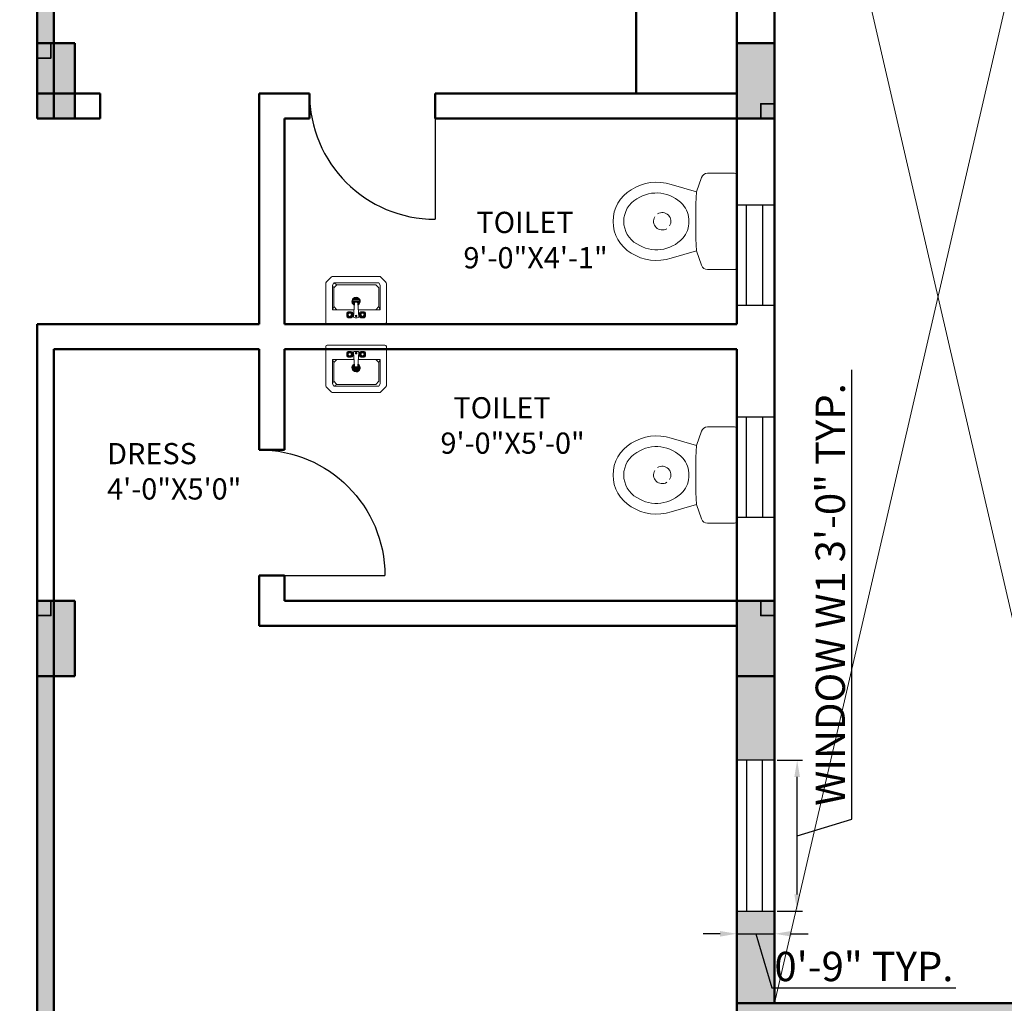
# Model space of a CAD drawing. Units: inches. Extents: x -7 to 1228, y -146 to 1091.
# Tile 63 of 88: x 376 to 611, y 655 to 890. Entities that reach past the tile are written whole.
import ezdxf

# ---------------------------------------------------------------- set-up
doc = ezdxf.new("R2010")
doc.units = ezdxf.units.IN
for name, color, linetype, lineweight in [('A-ANNO-DIMS', 2, 'Continuous', 18), ('A-AREA-IDEN', 7, 'Continuous', 18), ('A-COLS', 6, 'Continuous', 35), ('A-DOOR', 4, 'Continuous', 25), ('A-FLOR-FIXT', 8, 'Continuous', 18), ('A-FLOR-VOID', 7, 'Continuous', 18), ('A-FURN', 8, 'Continuous', 18), ('A-GLAZ', 175, 'Continuous', 25), ('A-WALL', 7, 'Continuous', 50), ('A-WALL-PATT', 251, 'Continuous', 13)]:
    doc.layers.add(name, color=color, linetype=linetype, lineweight=lineweight)
doc.styles.get("Standard").update_dxf_attribs({"font": 'arial.ttf'})
doc.dimstyles.new('ISO-25', dxfattribs={"dimtxt": 7, "dimasz": 4, "dimexe": 1.25, "dimexo": 0.625, "dimtad": 1, "dimdec": 1, "dimlunit": 3, "dimtxsty": 'Standard', "dimcen": 2.5, "dimadec": 0, "dimazin": 0, "dimtfac": 1, "dimtdec": 1, "dimtmove": 1, "dimatfit": 3, "dimfxl": 1, "dimarcsym": 0})

# ---------------------------------------------------------------- blocks, each defined once
blk = doc.blocks.new('A$C7B5C7CD4')
at = {"ltscale": 20}
for p, q in [((0, 0.614), (0, 0.4765)), ((0.243, 0.625), (0.011, 0.625)), ((0.243, 0.625), (0.475, 0.625)), ((0.486, 0.614), (0.486, 0.4765)), ((0.0212, 0.4467), (0.0946, 0.4214)), ((0.0946, 0.4214), (0.0576, 0.293)), ((0.0946, 0.4214), (0.1544, 0.4173)), ((0.3316, 0.4173), (0.1544, 0.4173)), ((0.3914, 0.4214), (0.3316, 0.4173)), ((0.4648, 0.4467), (0.3914, 0.4214)), ((0.3914, 0.4214), (0.4284, 0.293))]:
    blk.add_line(p, q, dxfattribs=at)
for centre, radius, start, end in [((0.011, 0.614), 0.011, 90, 180), ((0.475, 0.614), 0.011, 0, 90), ((0.0315, 0.4765), 0.0315, 180, 251), ((0.4545, 0.4765), 0.0315, 289, 0), ((0.2796, 0.219), 0.18, 132.4207, 213.289), ((0.24, 0.2602), 0.123, 88.6158, 131.7414), ((0.246, 0.2602), 0.123, 48.2586, 91.3842), ((0.2064, 0.219), 0.18, 326.711, 47.5793), ((0.2796, 0.219), 0.234, 161.5846, 212.8753), ((0.2064, 0.219), 0.234, 327.1247, 18.4154), ((0.243, 0.185), 0.131, 209.6292, 270), ((0.243, 0.185), 0.131, 270, 330.3708), ((0.243, 0.185), 0.185, 210.1745, 270), ((0.243, 0.185), 0.185, 270, 329.8255)]:
    blk.add_arc(centre, radius, start, end, dxfattribs=at)
for start, end in [(58.1785, 211.8215), (238.1785, 31.8215)]:
    blk.add_arc((0.2426, 0.2481), 0.0439, start, end)
blk = doc.blocks.new('A$C4CB854FF')
for p, q in [((0, 0.3675), (0, 0.0552)), ((0.4725, 0.38), (0.0125, 0.38)), ((0.1677, 0.2932), (0.1677, 0.318)), ((0.1745, 0.2919), (0.1745, 0.3194)), ((0.1773, 0.3221), (0.2048, 0.3221)), ((0.1787, 0.329), (0.2034, 0.329)), ((0.2075, 0.3194), (0.2075, 0.2919)), ((0.2144, 0.318), (0.2144, 0.2932)), ((0.2279, 0.2104), (0.2213, 0.3235)), ((0.2337, 0.329), (0.2502, 0.329)), ((0.2625, 0.3235), (0.256, 0.2104)), ((0.2694, 0.318), (0.2694, 0.2932)), ((0.2763, 0.3194), (0.2763, 0.2919)), ((0.3065, 0.3221), (0.279, 0.3221)), ((0.3052, 0.329), (0.2804, 0.329)), ((0.3093, 0.2919), (0.3093, 0.3194)), ((0.3162, 0.2932), (0.3162, 0.318)), ((0.485, 0.0552), (0.485, 0.3675)), ((0.05, 0.265), (0.2247, 0.265)), ((0.06, 0.24), (0.05, 0.265)), ((0.05, 0.07), (0.05, 0.265)), ((0.085, 0.265), (0.06, 0.24)), ((0.06, 0.24), (0.06, 0.09)), ((0.2048, 0.2891), (0.1773, 0.2891)), ((0.2034, 0.2822), (0.1787, 0.2822)), ((0.2591, 0.265), (0.43, 0.265)), ((0.279, 0.2891), (0.3065, 0.2891)), ((0.2804, 0.2822), (0.3052, 0.2822)), ((0.395, 0.265), (0.42, 0.24)), ((0.42, 0.24), (0.43, 0.265)), ((0.42, 0.24), (0.42, 0.09)), ((0.43, 0.07), (0.43, 0.265)), ((0.2152, 0.1984), (0.2694, 0.1984)), ((0.2297, 0.2066), (0.2165, 0.2066)), ((0.2681, 0.1901), (0.2165, 0.1901)), ((0.2272, 0.2149), (0.2208, 0.2149)), ((0.2638, 0.1819), (0.2208, 0.1819)), ((0.2533, 0.1736), (0.2313, 0.1736)), ((0.2505, 0.2052), (0.2334, 0.2052)), ((0.2681, 0.2066), (0.2541, 0.2066)), ((0.2638, 0.2149), (0.2566, 0.2149)), ((0.06, 0.09), (0.085, 0.065)), ((0.42, 0.09), (0.395, 0.065)), ((0.42, 0.09), (0.43, 0.07)), ((0.0037, 0.0463), (0.0463, 0.0037)), ((0.05, 0.07), (0.06, 0.05)), ((0.42, 0.05), (0.06, 0.05)), ((0.085, 0.065), (0.395, 0.065)), ((0.395, 0.065), (0.42, 0.05)), ((0.43, 0.07), (0.42, 0.05)), ((0.4387, 0.0037), (0.4813, 0.0463)), ((0.0552, 0), (0.4298, 0))]:
    blk.add_line(p, q)
for centre, radius in [((0.191, 0.3056), 0.0165), ((0.191, 0.3056), 0.0127), ((0.2419, 0.3152), 0.00688), ((0.2419, 0.3152), 0.00344), ((0.2928, 0.3056), 0.0165), ((0.2928, 0.3056), 0.0127)]:
    blk.add_circle(centre, radius)
for centre, radius, start, end in [((0.0125, 0.3675), 0.0125, 90, 180), ((0.1787, 0.318), 0.011, 90, 180), ((0.1773, 0.3194), 0.00275, 90, 180), ((0.2034, 0.318), 0.011, 0, 90), ((0.2048, 0.3194), 0.00275, 360, 90), ((0.2329, 0.314), 0.015, 87.19754, 140.72744), ((0.2509, 0.314), 0.015, 39.27256, 92.80246), ((0.2804, 0.318), 0.011, 90, 180), ((0.279, 0.3194), 0.00275, 90, 180), ((0.3052, 0.318), 0.011, 0, 90), ((0.3065, 0.3194), 0.00275, 360, 90), ((0.4725, 0.3675), 0.0125, 0, 90), ((0.1787, 0.2932), 0.011, 180, 270), ((0.1773, 0.2919), 0.00275, 180, 270), ((0.2034, 0.2932), 0.011, 270, 0), ((0.2048, 0.2919), 0.00275, 270, 0), ((0.2804, 0.2932), 0.011, 180, 270), ((0.279, 0.2919), 0.00275, 180, 270), ((0.3052, 0.2932), 0.011, 270, 360), ((0.3065, 0.2919), 0.00275, 270, 0), ((0.2423, 0.1984), 0.033, 118.68833, 62.86857), ((0.2423, 0.1984), 0.0271, 124.77581, 57.22467), ((0.2334, 0.2107), 0.0055, 183.3274, 270), ((0.2505, 0.2107), 0.0055, 270, 356.6726), ((0.0125, 0.0552), 0.0125, 180, 225), ((0.0552, 0.0125), 0.0125, 225, 270), ((0.4298, 0.0125), 0.0125, 270, 315), ((0.4725, 0.0552), 0.0125, 315, 0)]:
    blk.add_arc(centre, radius, start, end)
blk = doc.blocks.new('WIN-36')
for p, q in [((0, 36), (0, 0)), ((9, 36), (0, 36)), ((2.34, 36), (2.34, 0)), ((6.14, 0), (6.14, 36)), ((9, 0), (9, 36)), ((0, 0), (9, 0)), ((2.34, 0), (6.14, 0))]:
    blk.add_line(p, q)
blk = doc.blocks.new('WIN-24')
for p, q in [((0, 0), (0, 24)), ((0, 24), (9, 24)), ((2.34, 0), (2.34, 24)), ((2.34, 24), (6.14, 24)), ((6.14, 24), (6.14, 0)), ((9, 24), (9, 0)), ((9, 0), (0, 0))]:
    blk.add_line(p, q)
blk = doc.blocks.new('DOOR-750')
blk.add_line((30, 30), (30, 0))
blk.add_arc((30, 30), 30, 180, 270)
blk = doc.blocks.new('*D48')
at = {"layer": 'A-ANNO-DIMS', "color": 0, "lineweight": -2, "transparency": 16777216}
for p, q in [((574.46, 698.89), (574.46, 806.1)), ((556.62, 712.97), (562.65, 712.97)), ((561.4, 680.97), (561.4, 708.97)), ((561.4, 694.97), (574.46, 698.89)), ((556.62, 676.97), (562.65, 676.97))]:
    blk.add_line(p, q, dxfattribs=at)
at = {"layer": 'A-ANNO-DIMS', "color": 0, "transparency": 16777216}
for points in [[(560.73, 708.97), (562.07, 708.97), (561.4, 712.97)], [(560.73, 680.97), (562.07, 680.97), (561.4, 676.97)]]:
    blk.add_solid(points, dxfattribs=at)
at = {"layer": 'Defpoints', "color": 0, "transparency": 16777216}
for p in [(556, 712.97), (561.4, 712.97), (556, 676.97)]:
    blk.add_point(p, dxfattribs=at)
at = {"layer": 'A-ANNO-DIMS', "color": 0, "transparency": 16777216, "insert": (570.21, 752.49), "char_height": 7, "attachment_point": 5, "rotation": 90}
blk.add_mtext('WINDOW W1 3\'-0" TYP.', dxfattribs=at)
blk = doc.blocks.new('*D49')
at = {"layer": 'A-ANNO-DIMS', "color": 0, "lineweight": -2, "transparency": 16777216}
for p, q in [((547, 676.34), (547, 670.32)), ((556, 676.34), (556, 670.32)), ((543, 671.57), (539, 671.57)), ((547, 671.57), (556, 671.57)), ((547, 671.57), (556, 671.57)), ((551.5, 671.57), (555.37, 658.66)), ((560, 671.57), (564, 671.57)), ((555.37, 658.66), (599.29, 658.66))]:
    blk.add_line(p, q, dxfattribs=at)
at = {"layer": 'A-ANNO-DIMS', "color": 0, "transparency": 16777216}
for points in [[(543, 672.23), (543, 670.9), (547, 671.57)], [(560, 672.23), (560, 670.9), (556, 671.57)]]:
    blk.add_solid(points, dxfattribs=at)
at = {"layer": 'Defpoints', "color": 0, "transparency": 16777216}
for p in [(547, 676.97), (556, 676.97), (556, 671.57)]:
    blk.add_point(p, dxfattribs=at)
at = {"layer": 'A-ANNO-DIMS', "color": 0, "transparency": 16777216, "insert": (577.33, 662.86), "char_height": 7, "attachment_point": 5}
blk.add_mtext('0\'-9" TYP.', dxfattribs=at)

msp = doc.modelspace()

# ---------------------------------------------------------------- hatches: boundary and pattern name
at = {"layer": 'A-COLS'}
h = msp.add_hatch(color=256, dxfattribs=at)
h.dxf.hatch_style = 1
h.paths.add_polyline_path([(380, 866), (389, 866), (389, 884), (383.29, 884), (383.29, 880.45), (380, 880.45)])
h = msp.add_hatch(color=256, dxfattribs=at)
h.dxf.hatch_style = 1
h.paths.add_polyline_path([(383.29, 880.45), (383.29, 884), (380, 884), (380, 880.45)])
h = msp.add_hatch(color=256, dxfattribs=at)
h.dxf.hatch_style = 1
h.paths.add_polyline_path([(556, 884), (547, 884), (547, 866), (552.71, 866), (552.71, 869.55), (556, 869.55)])
h = msp.add_hatch(color=256, dxfattribs=at)
h.dxf.hatch_style = 1
h.paths.add_polyline_path([(552.71, 869.55), (552.71, 866), (556, 866), (556, 869.55)])
h = msp.add_hatch(color=256, dxfattribs=at)
h.dxf.hatch_style = 1
h.paths.add_polyline_path([(380, 733), (389, 733), (389, 751), (383.29, 751), (383.29, 747.45), (380, 747.45)])
h = msp.add_hatch(color=256, dxfattribs=at)
h.dxf.hatch_style = 1
h.paths.add_polyline_path([(383.29, 747.45), (383.29, 751), (380, 751), (380, 747.45)])
h = msp.add_hatch(color=256, dxfattribs=at)
h.dxf.hatch_style = 1
h.paths.add_polyline_path([(556, 747.45), (552.71, 747.45), (552.71, 751), (547, 751), (547, 733), (556, 733)])
h = msp.add_hatch(color=256, dxfattribs=at)
h.dxf.hatch_style = 1
h.paths.add_polyline_path([(556, 747.45), (556, 751), (552.71, 751), (552.71, 747.45)])
at = {"layer": 'A-WALL-PATT'}
h = msp.add_hatch(color=256, dxfattribs=at)
h.dxf.hatch_style = 1
h.paths.add_polyline_path([(69, 568), (60, 568), (60, 493), (63.29, 493), (69, 493)])
h.paths.add_polyline_path([(69, 662.41), (60, 662.41), (60, 586), (69, 586)], flags=17)
h.paths.add_polyline_path([(69, 723), (184, 723), (184, 734), (179, 734), (179, 728), (69, 728), (69, 741.62), (60, 741.62), (60, 698.41), (69, 698.41)], flags=17)
h.paths.add_polyline_path([(69, 782), (231, 782), (231, 728), (231, 723), (231, 586), (236, 586), (236, 787), (69, 787), (69, 800.13), (60, 800.13), (60, 765.62), (69, 765.62)])
h.paths.add_polyline_path([(184, 842), (189, 842), (189, 848), (173, 848), (173, 842), (179, 842), (179, 787), (184, 787)])
h.paths.add_polyline_path([(118.22, 69), (69, 69), (69, 60), (118.22, 60)])
h.paths.add_polyline_path([(227, 69), (154.22, 69), (154.22, 60), (227, 60)])
h.paths.add_polyline_path([(236, 60), (232.71, 60), (227, 60), (227, 36), (236, 36)])
h.paths.add_polyline_path([(389, 60), (380, 60), (380, 36), (389, 36)])
h.paths.add_polyline_path([(384, 181), (380, 181), (380, 115), (380, 78), (384, 78)])
h.paths.add_polyline_path([(380, 115), (334.55, 115), (334.55, 109), (380, 109)])
h.paths.add_polyline_path([(274.55, 115), (236, 115), (236, 201), (232.71, 201), (231, 201), (231, 78), (236, 78), (236, 109), (274.55, 109)])
h.paths.add_polyline_path([(69, 123), (60, 123), (60, 78), (69, 78)])
h.paths.add_polyline_path([(69, 201), (60, 201), (60, 159), (69, 159)])
h.paths.add_polyline_path([(143, 219), (69, 219), (69, 213), (143, 213)], flags=17)
h.paths.add_polyline_path([(189, 219), (184, 219), (184, 274), (231, 274), (231, 219), (236, 219), (236, 279), (184, 279), (184, 297), (179, 297), (179, 279), (69, 279), (69, 290.91), (60, 290.91), (60, 262.18), (69, 262.18), (69, 274), (179, 274), (179, 219), (173, 219), (173, 213), (189, 213)])
h.paths.add_polyline_path([(69, 238.18), (60, 238.18), (60, 219), (69, 219)], flags=17)
h.paths.add_polyline_path([(69, 333), (60, 333), (60, 314.91), (69, 314.91), (69, 316.96)])
h.paths.add_polyline_path([(190, 338), (184, 338), (69, 338), (69, 333), (179, 333), (179, 327), (184, 327), (184, 333.02), (190, 333.05)])
h.paths.add_polyline_path([(69, 386.81), (60, 386.81), (60, 351), (69, 351)])
h.paths.add_polyline_path([(69, 475), (60, 475), (60, 422.81), (69, 422.81)])
h.paths.add_polyline_path([(236, 475), (231, 475), (231, 351.24), (236, 351.24)])
h.paths.add_polyline_path([(384, 475), (380, 475), (380, 362), (384, 362)])
h.paths.add_polyline_path([(547, 307), (439, 307), (439, 356), (445, 356), (445, 362), (433, 362), (433, 307), (380, 307), (380, 244), (380, 241), (384, 241), (384, 301), (433, 301), (433, 277), (439, 277), (439, 301), (547, 301)])
h.paths.add_polyline_path([(547, 241), (439, 241), (439, 247), (433, 247), (433, 235), (547, 235)])
h.paths.add_polyline_path([(450, 69), (440.29, 69), (424.89, 69), (389, 69), (389, 60), (450, 60)])
h.paths.add_polyline_path([(547, 69), (486, 69), (486, 60), (547, 60)])
h.paths.add_polyline_path([(556, 148.27), (547, 148.27), (547, 78), (556, 78)])
h.paths.add_polyline_path([(556, 223), (547, 223), (547, 195), (547, 184.27), (556, 184.27)])
h.paths.add_polyline_path([(556, 311.19), (547, 311.19), (547, 273.08), (556, 273.08)])
h.paths.add_polyline_path([(556, 344), (552.71, 344), (547, 344), (547, 335.19), (556, 335.19)])
h.paths.add_polyline_path([(556, 249.08), (547, 249.08), (547, 241), (556, 241)])
h.paths.add_polyline_path([(547, 362), (475, 362), (475, 356), (547, 356)], flags=0)
h.paths.add_polyline_path([(556, 399.62), (547, 399.62), (547, 362), (556, 362)])
h.paths.add_polyline_path([(556, 475), (547, 475), (547, 435.62), (556, 435.62)])
h.paths.add_polyline_path([(547, 493), (389, 493), (389, 487), (547, 487)])
h.paths.add_polyline_path([(380, 493), (278, 493), (278, 487), (380, 487)])
h.paths.add_polyline_path([(227, 493), (69, 493), (69, 487), (227, 487)])
h.paths.add_polyline_path([(643, 122.44), (634, 122.44), (634, 78), (643, 78)])
h.paths.add_polyline_path([(702.5, 69), (692.79, 69), (677.39, 69), (643, 69), (643, 60), (702.5, 60)])
h.paths.add_polyline_path([(798, 69), (738.5, 69), (738.5, 60), (798, 60)])
h.paths.add_polyline_path([(807, 60), (803.71, 60), (798, 60), (798, 36), (807, 36)])
h.paths.add_polyline_path([(807, 109), (846.75, 109), (846.75, 115), (807, 115), (807, 159), (802, 159), (802, 78), (807, 78)])
h.paths.add_polyline_path([(807, 201), (802, 201), (802, 195), (807, 195)])
h.paths.add_polyline_path([(643, 201), (634, 201), (634, 158.44), (643, 158.44)])
h.paths.add_polyline_path([(756, 225), (751, 225), (751, 219), (643, 219), (643, 213), (756, 213)])
h.paths.add_polyline_path([(643, 240.85), (634, 240.85), (634, 219), (643, 219)])
h.paths.add_polyline_path([(643, 274), (643, 288.63), (634, 288.63), (634, 264.85), (643, 264.85)])
h.paths.add_polyline_path([(802, 279), (756, 279), (756, 297), (751, 297), (751, 279), (643, 279), (643, 274), (751, 274), (751, 255), (756, 255), (756, 274), (802, 274)])
h.paths.add_polyline_path([(807, 333), (803.71, 333), (802, 333), (802, 279), (802, 274), (802, 219), (807, 219)])
h.paths.add_polyline_path([(956, 182), (951, 182), (951, 115), (906.75, 115), (906.75, 109), (951, 109), (951, 78), (956, 78)])
h.paths.add_polyline_path([(960, 60), (951, 60), (951, 36), (960, 36)])
h.paths.add_polyline_path([(1021, 69), (1005.78, 69), (960, 69), (960, 60), (1021, 60)])
h.paths.add_polyline_path([(956, 224), (951, 224), (951, 218), (956, 218)])
h.paths.add_polyline_path([(956, 302), (1004, 302), (1004, 278), (1010, 278), (1010, 302), (1118, 302), (1118, 290.81), (1127, 290.81), (1127, 326.97), (1118, 326.97), (1118, 320.97), (1118, 307), (1010, 307), (1010, 356), (1016, 356), (1016, 362), (1004, 362), (1004, 307), (951, 307), (951, 244), (951, 242), (954.29, 242), (956, 242)])
h.paths.add_polyline_path([(643, 333), (634, 333), (634, 312.63), (643, 312.63), (643, 316.96)])
h.paths.add_polyline_path([(756, 338), (643, 338), (643, 333), (751, 333), (751, 327), (756, 327)])
h.paths.add_polyline_path([(643, 388), (634, 388), (634, 351), (643, 351)])
h.paths.add_polyline_path([(807, 357), (802, 357), (802, 351), (807, 351)])
h.paths.add_polyline_path([(807, 475), (802, 475), (802, 393), (807, 393)])
h.paths.add_polyline_path([(643, 475), (634, 475), (634, 424), (643, 424)])
h.paths.add_polyline_path([(798, 493), (643, 493), (643, 487), (798, 487)])
h.paths.add_polyline_path([(634, 493), (556, 493), (556, 487), (634, 487)])
h.paths.add_polyline_path([(813, 493), (807, 493), (807, 487), (813, 487)])
h.paths.add_polyline_path([(951, 493), (849, 493), (849, 487), (951, 487)])
h.paths.add_polyline_path([(956, 484), (951, 484), (951, 374), (956, 374)])
h.paths.add_polyline_path([(1109, 493), (969, 493), (969, 487), (1109, 487)])
h.paths.add_polyline_path([(1127, 484), (1118, 484), (1118, 450.64), (1127, 450.64)])
h.paths.add_polyline_path([(1127, 414.64), (1118, 414.64), (1118, 365), (1127, 365)])
h.paths.add_polyline_path([(1109, 362), (1046, 362), (1046, 356), (1109, 356)], flags=17)
h.paths.add_polyline_path([(1127, 356), (1123.45, 356), (1118, 356), (1118, 350.97), (1127, 350.97)], flags=0)
h.paths.add_polyline_path([(1127, 266.81), (1118, 266.81), (1118, 262.36), (1118, 242), (1127, 242)], flags=17)
h.paths.add_polyline_path([(1118, 242), (1010, 242), (1010, 248), (1004, 248), (1004, 237), (1118, 237)])
h.paths.add_polyline_path([(1127, 224), (1118, 224), (1118, 170), (1127, 170)])
h.paths.add_polyline_path([(1127, 134), (1118, 134), (1118, 78), (1127, 78)])
h.paths.add_polyline_path([(1118, 69), (1057, 69), (1057, 60), (1118, 60)])
h.paths.add_polyline_path([(227, 571.55), (227, 574), (69, 574), (69, 568), (227, 568)])
h.paths.add_polyline_path([(380, 571.55), (380, 574), (278, 574), (278, 568), (380, 568)])
h.paths.add_polyline_path([(242, 574), (236, 574), (236, 568), (242, 568)])
h.paths.add_polyline_path([(547, 571.55), (547, 574), (389, 574), (389, 568), (547, 568)])
h.paths.add_polyline_path([(384, 733), (380, 733), (380, 586), (384, 586)])
h.paths.add_polyline_path([(556, 646), (634, 646), (634, 655), (547, 655), (547, 586), (556, 586)])
h.paths.add_polyline_path([(634, 574), (556, 574), (556, 568), (634, 568)])
h.paths.add_polyline_path([(643, 655), (634, 655), (634, 586), (643, 586)])
h.paths.add_polyline_path([(798, 574), (643, 574), (643, 568), (798, 568)])
h.paths.add_polyline_path([(643, 663.85), (634, 663.85), (634, 655), (643, 655)])
h.paths.add_polyline_path([(556, 676.97), (547, 676.97), (547, 655), (556, 655)])
h.paths.add_polyline_path([(556, 733), (547, 733), (547, 712.97), (556, 712.97)])
h.paths.add_polyline_path([(643, 710), (634, 710), (634, 699.85), (643, 699.85)])
h.paths.add_polyline_path([(807, 668), (802, 668), (802, 586), (807, 586)])
h.paths.add_polyline_path([(951, 574), (849, 574), (849, 568), (951, 568)])
h.paths.add_polyline_path([(956, 691), (951, 691), (951, 577), (956, 577)])
h.paths.add_polyline_path([(1109, 574), (969, 574), (969, 568), (1109, 568)])
h.paths.add_polyline_path([(1127, 643.4), (1118, 643.4), (1118, 577), (1127, 577)])
h.paths.add_polyline_path([(1127, 568), (1123.45, 568), (1118, 568), (1118, 493), (1127, 493)])
h.paths.add_polyline_path([(1127, 733), (1118, 733), (1118, 679.4), (1127, 679.4)])
h.paths.add_polyline_path([(1127, 777.35), (1118, 777.35), (1118, 770.04), (1118, 751), (1127, 751)], flags=17)
h.paths.add_polyline_path([(1118, 751), (1010, 751), (1010, 757), (1004, 757), (1004, 745), (1118, 745)])
h.paths.add_polyline_path([(956, 811), (1004, 811), (1004, 787), (1010, 787), (1010, 811), (1017.87, 811), (1017.87, 811.63, -0.414214), (1018.25, 812), (1031.98, 812, -0.414214), (1032.35, 811.63), (1032.35, 811), (1118, 811), (1118, 801.35), (1127, 801.35), (1127, 834.69), (1118, 834.69), (1118, 830.24), (1118, 817), (1010, 817), (1010, 866), (1016, 866), (1016, 872), (1004, 872), (1004, 817), (956, 817), (956, 866), (951, 866), (951, 751), (954.29, 751), (956, 751)])
h.paths.add_polyline_path([(1118, 872), (1046, 872), (1046, 866), (1118, 866)], flags=17)
h.paths.add_polyline_path([(1127, 924.71), (1118, 924.71), (1118, 884), (1127, 884)])
h.paths.add_polyline_path([(1127, 866), (1123.71, 866), (1118, 866), (1118, 858.69), (1127, 858.69)], flags=17)
h.paths.add_polyline_path([(956, 983), (951, 983), (951, 952), (807, 952), (807, 983), (802, 983), (802, 902), (807, 902), (807, 946), (951, 946), (951, 884), (956, 884)])
h.paths.add_polyline_path([(807, 842), (802, 842), (802, 787), (756, 787), (756, 806), (751, 806), (751, 787), (643, 787), (643, 782), (751, 782), (751, 764), (756, 764), (756, 782), (802, 782), (802, 728), (807, 728)])
h.paths.add_polyline_path([(756, 848), (643, 848), (643, 842), (751, 842), (751, 836), (756, 836)])
h.paths.add_polyline_path([(756, 734), (751, 734), (751, 728), (643, 728), (643, 723), (756, 723)])
h.paths.add_polyline_path([(643, 749.79), (634, 749.79), (634, 728), (637.29, 728), (643, 728)])
h.paths.add_polyline_path([(643, 805.41), (634, 805.41), (634, 773.79), (643, 773.79)])
h.paths.add_polyline_path([(643, 896.66), (634, 896.66), (634, 860), (637.29, 860), (643, 860)])
h.paths.add_polyline_path([(643, 842), (634, 842), (634, 829.41), (643, 829.41)])
h.paths.add_polyline_path([(643, 983), (634, 983), (634, 932.66), (643, 932.66)])
h.paths.add_polyline_path([(1127, 983), (1118, 983), (1118, 960.71), (1127, 960.71)])
h.paths.add_polyline_path([(1118, 1001), (1077.53, 1001), (1077.53, 992), (1118, 992)])
h.paths.add_polyline_path([(1041.53, 1001), (960, 1001), (960, 992), (1041.53, 992)])
h.paths.add_polyline_path([(960, 1025), (951, 1025), (951, 1001), (954.29, 1001), (960, 1001)])
h.paths.add_polyline_path([(807, 1025), (798, 1025), (798, 1001), (807, 1001)])
h.paths.add_polyline_path([(798, 1001), (738.5, 1001), (738.5, 992), (798, 992)])
h.paths.add_polyline_path([(702.5, 1001), (643, 1001), (643, 992), (702.5, 992)])
h.paths.add_polyline_path([(547, 1001), (499.11, 1001), (499.11, 992), (547, 992)])
h.paths.add_polyline_path([(463.11, 1001), (389, 1001), (389, 992), (463.11, 992)])
h.paths.add_polyline_path([(389, 1025), (380, 1025), (380, 1022), (380, 1001), (383.29, 1001), (389, 1001)])
h.paths.add_polyline_path([(236, 1025), (227, 1025), (227, 1001), (236, 1001)])
h.paths.add_polyline_path([(236, 983), (231, 983), (231, 860), (236, 860)])
h.paths.add_polyline_path([(274.55, 952), (236, 952), (236, 946), (274.55, 946)])
h.paths.add_polyline_path([(380, 952), (334.55, 952), (334.55, 946), (380, 946)])
h.paths.add_polyline_path([(384, 983), (380, 983), (380, 884), (383.29, 884), (384, 884)])
h.paths.add_polyline_path([(227, 1001), (155.01, 1001), (155.01, 992), (162.87, 992), (227, 992)])
h.paths.add_polyline_path([(119.01, 1001), (69, 1001), (69, 992), (119.01, 992)])
h.paths.add_polyline_path([(69, 983), (60, 983), (60, 922.99), (69, 922.99)])
h.paths.add_polyline_path([(69, 886.99), (60, 886.99), (60, 860), (63.29, 860), (69, 860)])
h.paths.add_polyline_path([(143, 848), (69, 848), (69, 842), (143, 842)])

# ---------------------------------------------------------------- linework, layer by layer
at = {"layer": 'A-COLS'}
for points in [[(380, 884), (383.29, 884), (383.29, 880.45), (380, 880.45)], [(556, 866), (552.71, 866), (552.71, 869.55), (556, 869.55)], [(380, 751), (383.29, 751), (383.29, 747.45), (380, 747.45)], [(556, 751), (552.71, 751), (552.71, 747.45), (556, 747.45)]]:
    msp.add_lwpolyline(points, close=True, dxfattribs=at)
at = {"layer": 'A-FLOR-VOID'}
for p, q in [((556, 992), (634, 655)), ((556, 655), (634, 991.66))]:
    msp.add_line(p, q, dxfattribs=at)
at = {"layer": 'A-WALL'}
for p, q in [((380, 1001), (380, 866)), ((384, 1001), (384, 866)), ((547, 1001), (547, 872)), ((556, 1001), (556, 655)), ((523, 968), (523, 872)), ((380, 884), (389, 884)), ((380, 866), (380, 884)), ((389, 884), (389, 866)), ((547, 866), (547, 884)), ((547, 884), (556, 884)), ((556, 884), (556, 866)), ((395, 872), (380, 872)), ((389, 866), (389, 872)), ((395, 866), (395, 872)), ((433, 872), (433, 817)), ((445, 872), (433, 872)), ((445, 866), (445, 872)), ((547, 872), (475, 872)), ((475, 866), (475, 872)), ((389, 866), (380, 866)), ((395, 866), (380, 866)), ((439, 866), (439, 817)), ((445, 866), (439, 866)), ((547, 866), (475, 866)), ((547, 866), (547, 817)), ((556, 866), (547, 866)), ((380, 817), (380, 574)), ((433, 817), (380, 817)), ((547, 817), (439, 817)), ((384, 811), (384, 574)), ((433, 811), (384, 811)), ((433, 811), (433, 787)), ((547, 811), (439, 811)), ((439, 811), (439, 787)), ((547, 811), (547, 751)), ((439, 787), (433, 787)), ((439, 757), (433, 757)), ((433, 757), (433, 745)), ((439, 757), (439, 751)), ((380, 751), (389, 751)), ((380, 733), (380, 751)), ((389, 751), (389, 733)), ((547, 751), (439, 751)), ((556, 751), (547, 751)), ((547, 751), (547, 733)), ((556, 733), (556, 751)), ((547, 745), (433, 745)), ((547, 745), (547, 574)), ((389, 733), (389, 739)), ((389, 733), (380, 733)), ((547, 733), (556, 733)), ((643, 655), (547, 655))]:
    msp.add_line(p, q, dxfattribs=at)

# ---------------------------------------------------------------- block references
at = {"layer": 'A-DOOR'}
msp.add_blockref('DOOR-750', (445, 842), dxfattribs=at)
at = {"layer": 'A-DOOR', "extrusion": (0, 0, -1), "zscale": -1, "rotation": 269.9999999999998}
msp.add_blockref('DOOR-750', (-463, 787), dxfattribs=at)
at = {"layer": 'A-FLOR-FIXT', "xscale": 47.26153857112405, "yscale": 47.26153857112405, "zscale": 47.26153857112405, "rotation": 270}
for p in [(517.46, 852.98), (517.46, 792.48)]:
    msp.add_blockref('A$C7B5C7CD4', p, dxfattribs=at)
at = {"layer": 'A-FURN', "xscale": 29.84864686937646, "yscale": 29.84864686937646, "zscale": 29.84864686937646, "rotation": 180}
msp.add_blockref('A$C4CB854FF', (463.35, 828.34), dxfattribs=at)
at = {"layer": 'A-FURN', "xscale": -29.84864686937646, "yscale": 29.84864686937646, "zscale": 29.84864686937646}
msp.add_blockref('A$C4CB854FF', (463.35, 800.66), dxfattribs=at)
at = {"layer": 'A-GLAZ'}
for name, p in [('WIN-24', (547, 821.43)), ('WIN-24', (547, 770.86)), ('WIN-36', (547, 676.97))]:
    msp.add_blockref(name, p, dxfattribs=at)

# ---------------------------------------------------------------- texts
at = {"layer": 'A-AREA-IDEN', "attachment_point": 1}
for s, insert, char_height in [('  TOILET\\P9\'-0"X4\'-1"', (481.74, 843.78), 5.0568), ('  TOILET\\P9\'-0"X5\'-0"', (476.26, 799.56), 5.0568), ('DRESS\\P4\'-0"X5\'0"', (396.7, 788.63), 5.057)]:
    msp.add_mtext_dynamic_manual_height_columns(s, width=137.2821, gutter_width=25.28, heights=[0], dxfattribs=dict(at, insert=insert, char_height=char_height))

# ---------------------------------------------------------------- dimensions: what is measured, and where the dimension line sits
at = {"layer": 'A-ANNO-DIMS'}
dim = msp.add_linear_dim(base=(561.4, 712.97), p1=(556, 676.97), p2=(556, 712.97), angle=90, text='WINDOW W1 <> TYP.', dimstyle='ISO-25', override={"dimdec": 1, "dimlfac": 1, "dimrnd": 0, "dimzin": 1, "dimdsep": 46, "dimlunit": 4, "dimfrac": 2}, dxfattribs=at)
dim.commit()
dim.dimension.update_dxf_attribs({"geometry": '*D48', "text_midpoint": (570.21, 699.51)})
dim = msp.add_linear_dim(base=(556, 671.57), p1=(547, 676.97), p2=(556, 676.97), text='<> TYP.', dimstyle='ISO-25', override={"dimdec": 1, "dimlfac": 1, "dimrnd": 0, "dimzin": 1, "dimdsep": 46, "dimlunit": 4, "dimfrac": 2}, dxfattribs=at)
dim.commit()
dim.dimension.update_dxf_attribs({"geometry": '*D49', "text_midpoint": (556, 662.86)})

doc.saveas('drawing.dxf')
